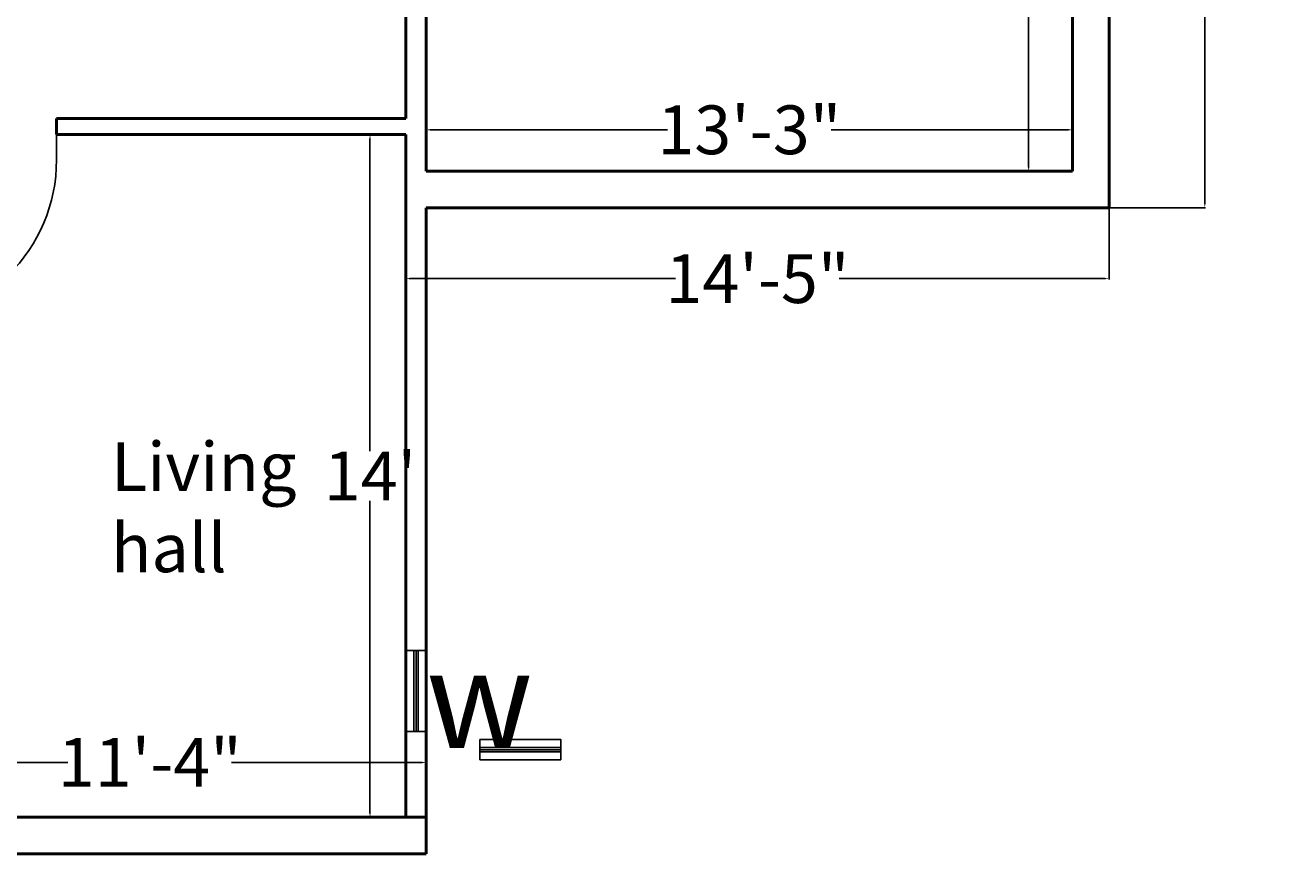
# Model space of a CAD drawing. Units: inches. Extents: x 409 to 7572, y 7 to 725.
# Tile 5 of 38: x 860 to 1171, y 157 to 360. Entities that reach past the tile are written whole.
import ezdxf

# ---------------------------------------------------------------- set-up
doc = ezdxf.new("R2010")
doc.units = ezdxf.units.IN
doc.header["$MEASUREMENT"] = 0
for name, color, linetype, lineweight in [('A-ANNO-DIMS', 2, 'Continuous', 18), ('A-ANNO-SYMB', 3, 'Continuous', 25), ('A-AREA-IDEN', 7, 'Continuous', 25), ('A-DOOR', 3, 'Continuous', 25), ('A-GLAZ', 4, 'Continuous', 25), ('A-WALL', 7, 'Continuous', 50)]:
    doc.layers.add(name, color=color, linetype=linetype, lineweight=lineweight)
doc.styles.get("Standard").update_dxf_attribs({"font": 'arial.ttf'})
doc.dimstyles.get("Standard").update_dxf_attribs({"dimtxt": 2, "dimasz": 1, "dimexe": 0.18, "dimexo": 0.0625, "dimgap": 0.09, "dimtad": 0, "dimtih": 1, "dimtoh": 1, "dimdec": 0, "dimzin": 0, "dimdsep": 46, "dimlunit": 3, "dimtxsty": 'Standard', "dimcen": 0.09, "dimadec": 0, "dimazin": 0, "dimtfac": 1, "dimtdec": 0, "dimtofl": 0, "dimtmove": 0, "dimatfit": 3, "dimfxl": 1, "dimtolj": 1, "dimtzin": 0, "dimarcsym": 0})

# ---------------------------------------------------------------- blocks, each defined once
blk = doc.blocks.new('*U5')
for p, q in [((0, 0), (0, 6)), ((40, 0), (40, 6))]:
    blk.add_line(p, q)
blk.add_lwpolyline([(0, 0), (0, -40), (1.75, -40), (1.75, 0)], close=True)
blk.add_arc((0, 0), 40, 270, 0)
blk = doc.blocks.new('*D13')
at = {"layer": 'A-ANNO-DIMS', "color": 0, "lineweight": -2, "transparency": 16777216}
for p, q in [((1117.09, 444.53), (1106.21, 444.53)), ((1106.39, 443.53), (1106.39, 390.75)), ((1106.39, 325.53), (1106.39, 378.31)), ((1117.09, 324.53), (1106.21, 324.53))]:
    blk.add_line(p, q, dxfattribs=at)
at = {"layer": 'A-ANNO-DIMS', "color": 0, "transparency": 16777216}
for points in [[(1106.22, 443.53), (1106.56, 443.53), (1106.39, 444.53)], [(1106.22, 325.53), (1106.56, 325.53), (1106.39, 324.53)]]:
    blk.add_solid(points, dxfattribs=at)
at = {"layer": 'DEFPOINTS', "color": 0, "transparency": 16777216}
for p in [(1106.39, 444.53), (1117.16, 444.53), (1117.16, 324.53)]:
    blk.add_point(p, dxfattribs=at)
at = {"layer": 'A-ANNO-DIMS', "color": 0, "transparency": 16777216, "insert": (1106.39, 384.53), "char_height": 2, "attachment_point": 5}
blk.add_mtext("\\A1;{\\H6x;10'}", dxfattribs=at)
blk = doc.blocks.new('*D14')
at = {"layer": 'A-ANNO-DIMS', "color": 0, "lineweight": -2, "transparency": 16777216}
for p, q in [((958.16, 324.59), (958.16, 334.9)), ((959.16, 334.72), (1017.52, 334.72)), ((1116.16, 334.72), (1057.79, 334.72)), ((1117.16, 324.59), (1117.16, 334.9))]:
    blk.add_line(p, q, dxfattribs=at)
at = {"layer": 'A-ANNO-DIMS', "color": 0, "transparency": 16777216}
for points in [[(959.16, 334.88), (959.16, 334.55), (958.16, 334.72)], [(1116.16, 334.88), (1116.16, 334.55), (1117.16, 334.72)]]:
    blk.add_solid(points, dxfattribs=at)
at = {"layer": 'DEFPOINTS', "color": 0, "transparency": 16777216}
for p in [(958.16, 334.72), (958.16, 324.53), (1117.16, 324.53)]:
    blk.add_point(p, dxfattribs=at)
at = {"layer": 'A-ANNO-DIMS', "color": 0, "transparency": 16777216, "insert": (1037.66, 334.72), "char_height": 2, "attachment_point": 5}
blk.add_mtext('\\A1;{\\H6x;13\'-3"}', dxfattribs=at)
blk = doc.blocks.new('*D15')
at = {"layer": 'A-ANNO-DIMS', "color": 0, "lineweight": -2, "transparency": 16777216}
for p, q in [((953.09, 333.53), (944.16, 333.53)), ((944.34, 332.53), (944.34, 255.65)), ((944.34, 166.53), (944.34, 243.42)), ((953.09, 165.53), (944.16, 165.53))]:
    blk.add_line(p, q, dxfattribs=at)
at = {"layer": 'A-ANNO-DIMS', "color": 0, "transparency": 16777216}
for points in [[(944.18, 332.53), (944.51, 332.53), (944.34, 333.53)], [(944.18, 166.53), (944.51, 166.53), (944.34, 165.53)]]:
    blk.add_solid(points, dxfattribs=at)
at = {"layer": 'DEFPOINTS', "color": 0, "transparency": 16777216}
for p in [(953.16, 333.53), (944.34, 165.53), (953.16, 165.53)]:
    blk.add_point(p, dxfattribs=at)
at = {"layer": 'A-ANNO-DIMS', "color": 0, "transparency": 16777216, "insert": (944.34, 249.53), "char_height": 2, "attachment_point": 5}
blk.add_mtext("\\A1;{\\H6x;14'}", dxfattribs=at)
blk = doc.blocks.new('*D16')
at = {"layer": 'A-ANNO-DIMS', "color": 0, "lineweight": -2, "transparency": 16777216}
for p, q in [((822.16, 165.59), (822.16, 179.18)), ((823.16, 179), (870.02, 179)), ((957.16, 179), (910.29, 179)), ((958.16, 165.59), (958.16, 179.18))]:
    blk.add_line(p, q, dxfattribs=at)
at = {"layer": 'A-ANNO-DIMS', "color": 0, "transparency": 16777216}
for points in [[(823.16, 179.16), (823.16, 178.83), (822.16, 179)], [(957.16, 179.16), (957.16, 178.83), (958.16, 179)]]:
    blk.add_solid(points, dxfattribs=at)
at = {"layer": 'DEFPOINTS', "color": 0, "transparency": 16777216}
for p in [(958.16, 179), (822.16, 165.53), (958.16, 165.53)]:
    blk.add_point(p, dxfattribs=at)
at = {"layer": 'A-ANNO-DIMS', "color": 0, "transparency": 16777216, "insert": (890.16, 179), "char_height": 2, "attachment_point": 5}
blk.add_mtext('\\A1;{\\H6x;11\'-4"}', dxfattribs=at)
blk = doc.blocks.new('*D35')
at = {"layer": 'A-ANNO-DIMS', "color": 0, "lineweight": -2, "transparency": 16777216}
for p, q in [((1126.22, 672.53), (1149.9, 672.53)), ((1149.72, 671.53), (1149.72, 500.86)), ((1149.72, 316.53), (1149.72, 488.43)), ((1126.22, 315.53), (1149.9, 315.53))]:
    blk.add_line(p, q, dxfattribs=at)
at = {"layer": 'A-ANNO-DIMS', "color": 0, "transparency": 16777216}
for points in [[(1149.56, 671.53), (1149.89, 671.53), (1149.72, 672.53)], [(1149.56, 316.53), (1149.89, 316.53), (1149.72, 315.53)]]:
    blk.add_solid(points, dxfattribs=at)
at = {"layer": 'DEFPOINTS', "color": 0, "transparency": 16777216}
for p in [(1126.16, 672.53), (1149.72, 672.53), (1126.16, 315.53)]:
    blk.add_point(p, dxfattribs=at)
at = {"layer": 'A-ANNO-DIMS', "color": 0, "transparency": 16777216, "insert": (1149.72, 494.65), "char_height": 2, "attachment_point": 5}
blk.add_mtext('\\A1;{\\H6x;29\'-9"}', dxfattribs=at)
blk = doc.blocks.new('*D36')
at = {"layer": 'A-ANNO-DIMS', "color": 0, "lineweight": -2, "transparency": 16777216}
for p, q in [((953.16, 315.37), (953.16, 297.9)), ((1126.16, 315.37), (1126.16, 297.9)), ((954.16, 298.08), (1019.52, 298.08)), ((1125.16, 298.08), (1059.79, 298.08))]:
    blk.add_line(p, q, dxfattribs=at)
at = {"layer": 'A-ANNO-DIMS', "color": 0, "transparency": 16777216}
for points in [[(954.16, 298.25), (954.16, 297.92), (953.16, 298.08)], [(1125.16, 298.25), (1125.16, 297.92), (1126.16, 298.08)]]:
    blk.add_solid(points, dxfattribs=at)
at = {"layer": 'DEFPOINTS', "color": 0, "transparency": 16777216}
for p in [(953.16, 315.43), (1126.16, 315.43), (1126.16, 298.08)]:
    blk.add_point(p, dxfattribs=at)
at = {"layer": 'A-ANNO-DIMS', "color": 0, "transparency": 16777216, "insert": (1039.66, 298.08), "char_height": 2, "attachment_point": 5}
blk.add_mtext('\\A1;{\\H6x;14\'-5"}', dxfattribs=at)
blk = doc.blocks.new('WIN-20')
for p, q in [((2103.48, 182.68), (2083.54, 182.68)), ((2103.48, 182.13), (2083.54, 182.13)), ((2103.48, 181.57), (2083.54, 181.57))]:
    blk.add_line(p, q)
blk.add_lwpolyline([(2103.48, 179.64), (2083.54, 179.64), (2083.54, 184.62), (2103.48, 184.62)], close=True)

msp = doc.modelspace()

# ---------------------------------------------------------------- linework, layer by layer
at = {"layer": 'A-WALL'}
for p, q in [((1126.16, 315.53), (1126.16, 672.53)), ((953.16, 525.53), (953.16, 337.53)), ((953.16, 489.53), (953.16, 337.53)), ((958.16, 444.53), (958.16, 324.53)), ((1117.16, 324.53), (1117.16, 444.53)), ((867.22, 337.53), (867.22, 333.53)), ((867.22, 337.53), (953.16, 337.53)), ((867.22, 333.53), (953.16, 333.53)), ((953.16, 333.53), (953.16, 165.53)), ((953.16, 333.53), (953.16, 165.53)), ((1117.16, 324.53), (958.16, 324.53)), ((1126.16, 315.53), (958.16, 315.53)), ((958.16, 315.53), (958.16, 165.53)), ((822.16, 165.53), (958.16, 165.53)), ((958.16, 165.53), (958.16, 156.53)), ((584.16, 156.53), (958.16, 156.53))]:
    msp.add_line(p, q, dxfattribs=at)

# ---------------------------------------------------------------- block references
at = {"layer": 'A-DOOR'}
msp.add_blockref('*U5', (827.22, 327.37), dxfattribs=at)
at = {"layer": 'A-GLAZ', "rotation": 89.99999999999905}
msp.add_blockref('WIN-20', (1137.79, -1896.94), dxfattribs=at)
at = {"layer": 'A-GLAZ'}
msp.add_blockref('WIN-20', (-1112.16, 0), dxfattribs=at)

# ---------------------------------------------------------------- texts
at = {"layer": 'A-ANNO-SYMB', "insert": (958.16, 206.54), "char_height": 24, "attachment_point": 1}
msp.add_mtext_dynamic_manual_height_columns('w', width=18.2582, gutter_width=1, heights=[0], dxfattribs=at)
at = {"layer": 'A-AREA-IDEN', "insert": (880.62, 257.83), "char_height": 12, "attachment_point": 1}
msp.add_mtext_dynamic_manual_height_columns('Living hall', width=58.8843, gutter_width=1, heights=[0], dxfattribs=at)

# ---------------------------------------------------------------- dimensions: what is measured, and where the dimension line sits
at = {"layer": 'A-ANNO-DIMS'}
dim = msp.add_linear_dim(base=(1149.72, 672.53), p1=(1126.16, 315.53), p2=(1126.16, 672.53), angle=90, text='{\\H6x;<>}', dimstyle='Standard', override={"dimclrd": 0, "dimclre": 0, "dimclrt": 0}, dxfattribs=at)
dim.commit()
dim.dimension.update_dxf_attribs({"geometry": '*D35', "text_midpoint": (1149.72, 494.65), "dimtype": 160})
for base, p1, p2, picture, middle in [((1106.39, 444.53), (1117.16, 324.53), (1117.16, 444.53), '*D13', (1106.39, 384.53)), ((944.34, 165.53), (953.16, 333.53), (953.16, 165.53), '*D15', (944.34, 249.53))]:
    dim = msp.add_linear_dim(base=base, p1=p1, p2=p2, angle=90, text='{\\H6x;<>}', dimstyle='Standard', override={"dimclrd": 0, "dimclre": 0, "dimclrt": 0}, dxfattribs=at)
    dim.commit()
    dim.dimension.update_dxf_attribs({"geometry": picture, "text_midpoint": middle})
for base, p1, p2, picture, middle in [((958.16, 334.72), (1117.16, 324.53), (958.16, 324.53), '*D14', (1037.66, 334.72)), ((1126.16, 298.08), (953.16, 315.43), (1126.16, 315.43), '*D36', (1039.66, 298.08)), ((958.16, 179), (822.16, 165.53), (958.16, 165.53), '*D16', (890.16, 179))]:
    dim = msp.add_linear_dim(base=base, p1=p1, p2=p2, text='{\\H6x;<>}', dimstyle='Standard', override={"dimclrd": 0, "dimclre": 0, "dimclrt": 0}, dxfattribs=at)
    dim.commit()
    dim.dimension.update_dxf_attribs({"geometry": picture, "text_midpoint": middle})

doc.saveas('drawing.dxf')
